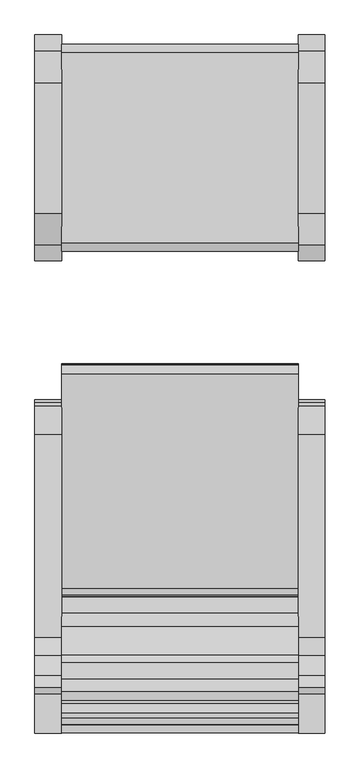
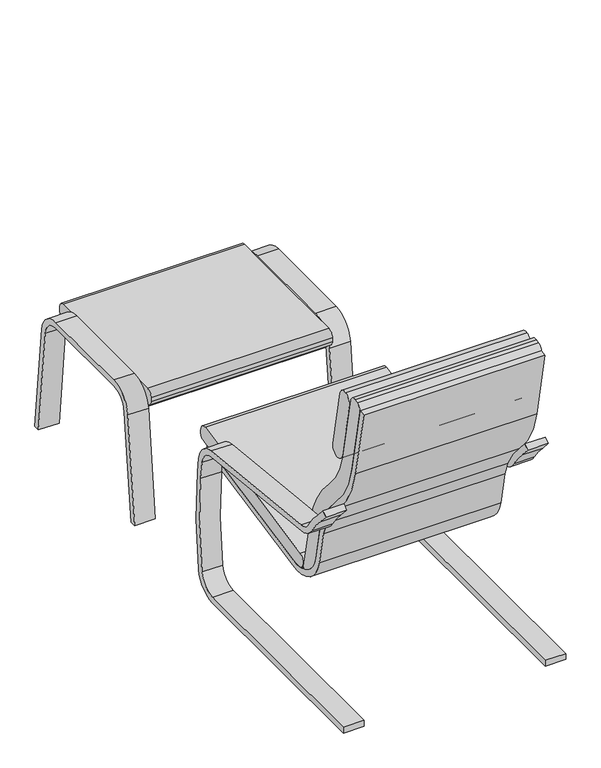
"""IFC4 building model written with IfcOpenShell, lengths in millimetres: furniture geometry."""

from ifc_helpers import new_model, si_unit, point, frame, frame_2d, origin, place, context, project, spatial, polyline, circle_curve, trimmed, segment, composite_curve, outline, extrude, source, transform, mapped, element, save


def furniture_b0964881(model_context):
    return source(origin(), model_context, "Body", "SweptSolid", [
        extrude(outline(composite_curve([segment(polyline([(-419.1, 19.05), (279.4542155, 19.05)]), True, "CONTINUOUS"), segment(trimmed(circle_curve(frame_2d((279.4542155, 76.2)), 57.15), [point((279.4542155, 19.05))], [point((335.932198, 67.4615796))], True, "CARTESIAN"), True, "CONTINUOUS"), segment(trimmed(circle_curve(frame_2d((-796.2501085, 242.6357718)), 1145.6538626), [point((335.932198, 67.4615796))], [point((342.5646303, 367.6308255))], True, "CARTESIAN"), True, "CONTINUOUS"), segment(trimmed(circle_curve(frame_2d((-796.2501085, 242.6357718)), 1145.6538626), [point((342.5646303, 367.6308255))], [point((334.8764989, 424.5021261))], True, "CARTESIAN"), True, "CONTINUOUS"), segment(trimmed(circle_curve(frame_2d((278.4511791, 415.4298727)), 57.15), [point((334.8764989, 424.5021261))], [point((284.4291769, 472.2663579))], True, "CARTESIAN"), True, "CONTINUOUS"), segment(polyline([(284.4291769, 472.2663579), (-194.9045529, 522.682143)]), True, "CONTINUOUS"), segment(trimmed(circle_curve(frame_2d((-186.9338891, 598.4641231)), 76.2), [point((-194.9045529, 522.682143))], [point((-251.8204957, 558.5120484))], False, "CARTESIAN"), True, "CONTINUOUS"), segment(trimmed(circle_curve(frame_2d((-499.260365, 406.1580161)), 290.5825873), [point((-251.8204957, 558.5120484))], [point((-296.3293666, 614.1417893))], True, "CARTESIAN"), True, "CONTINUOUS"), segment(trimmed(circle_curve(frame_2d((-56.8620262, 859.5716222)), 342.9), [point((-296.3293666, 614.1417893))], [point((-326.0096311, 647.1099157))], False, "CARTESIAN"), True, "CONTINUOUS"), segment(polyline([(-326.0096311, 647.1099157), (-311.0569864, 658.9133438)]), True, "CONTINUOUS"), segment(trimmed(circle_curve(frame_2d((-56.8620262, 859.5716222)), 323.85), [point((-311.0569864, 658.9133438))], [point((-283.0256254, 627.7767801))], True, "CARTESIAN"), True, "CONTINUOUS"), segment(trimmed(circle_curve(frame_2d((-499.260365, 406.1580161)), 309.6325873), [point((-283.0256254, 627.7767801))], [point((-235.598844, 568.500067))], False, "CARTESIAN"), True, "CONTINUOUS"), segment(trimmed(circle_curve(frame_2d((-186.9338891, 598.4641231)), 57.15), [point((-235.598844, 568.500067))], [point((-192.9118869, 541.627638))], True, "CARTESIAN"), True, "CONTINUOUS"), segment(polyline([(-192.9118869, 541.627638), (286.4218429, 491.2118529)]), True, "CONTINUOUS"), segment(trimmed(circle_curve(frame_2d((278.4511791, 415.4298727)), 76.2), [point((286.4218429, 491.2118529))], [point((353.6849388, 427.5262106))], False, "CARTESIAN"), True, "CONTINUOUS"), segment(trimmed(circle_curve(frame_2d((-796.2501085, 242.6357718)), 1164.7038626), [point((353.6849388, 427.5262106))], [point((360.5049853, 378.4766361))], False, "CARTESIAN"), True, "CONTINUOUS"), segment(trimmed(circle_curve(frame_2d((-796.2501085, 242.6357718)), 1164.7038626), [point((360.5049853, 378.4766361))], [point((354.7581922, 64.5487728))], False, "CARTESIAN"), True, "CONTINUOUS"), segment(trimmed(circle_curve(frame_2d((279.4542155, 76.2)), 76.2), [point((354.7581922, 64.5487728))], [point((279.4542155, 0.0))], False, "CARTESIAN"), True, "CONTINUOUS"), segment(polyline([(279.4542155, 0.0), (-419.1, 0.0), (-419.1, 19.05)]), True, "CONTINUOUS")], self_intersect=False)), frame((279.4, 0.0, 0.0), z_axis=(1.0, 0.0, 0.0), x_axis=(0.0, 1.0, 0.0)), (0.0, 0.0, 1.0), 63.5),
        extrude(outline(composite_curve([segment(polyline([(-419.1, 19.05), (279.4542155, 19.05)]), True, "CONTINUOUS"), segment(trimmed(circle_curve(frame_2d((279.4542155, 76.2)), 57.15), [point((279.4542155, 19.05))], [point((335.932198, 67.4615796))], True, "CARTESIAN"), True, "CONTINUOUS"), segment(trimmed(circle_curve(frame_2d((-796.2501085, 242.6357718)), 1145.6538626), [point((335.932198, 67.4615796))], [point((342.5646303, 367.6308255))], True, "CARTESIAN"), True, "CONTINUOUS"), segment(trimmed(circle_curve(frame_2d((-796.2501085, 242.6357718)), 1145.6538626), [point((342.5646303, 367.6308255))], [point((334.8764989, 424.5021261))], True, "CARTESIAN"), True, "CONTINUOUS"), segment(trimmed(circle_curve(frame_2d((278.4511791, 415.4298727)), 57.15), [point((334.8764989, 424.5021261))], [point((284.4291769, 472.2663579))], True, "CARTESIAN"), True, "CONTINUOUS"), segment(polyline([(284.4291769, 472.2663579), (-194.9045529, 522.682143)]), True, "CONTINUOUS"), segment(trimmed(circle_curve(frame_2d((-186.9338891, 598.4641231)), 76.2), [point((-194.9045529, 522.682143))], [point((-251.8204957, 558.5120484))], False, "CARTESIAN"), True, "CONTINUOUS"), segment(trimmed(circle_curve(frame_2d((-499.260365, 406.1580161)), 290.5825873), [point((-251.8204957, 558.5120484))], [point((-296.3293666, 614.1417893))], True, "CARTESIAN"), True, "CONTINUOUS"), segment(trimmed(circle_curve(frame_2d((-56.8620262, 859.5716222)), 342.9), [point((-296.3293666, 614.1417893))], [point((-326.0096311, 647.1099157))], False, "CARTESIAN"), True, "CONTINUOUS"), segment(polyline([(-326.0096311, 647.1099157), (-311.0569864, 658.9133438)]), True, "CONTINUOUS"), segment(trimmed(circle_curve(frame_2d((-56.8620262, 859.5716222)), 323.85), [point((-311.0569864, 658.9133438))], [point((-283.0256254, 627.7767801))], True, "CARTESIAN"), True, "CONTINUOUS"), segment(trimmed(circle_curve(frame_2d((-499.260365, 406.1580161)), 309.6325873), [point((-283.0256254, 627.7767801))], [point((-235.598844, 568.500067))], False, "CARTESIAN"), True, "CONTINUOUS"), segment(trimmed(circle_curve(frame_2d((-186.9338891, 598.4641231)), 57.15), [point((-235.598844, 568.500067))], [point((-192.9118869, 541.627638))], True, "CARTESIAN"), True, "CONTINUOUS"), segment(polyline([(-192.9118869, 541.627638), (286.4218429, 491.2118529)]), True, "CONTINUOUS"), segment(trimmed(circle_curve(frame_2d((278.4511791, 415.4298727)), 76.2), [point((286.4218429, 491.2118529))], [point((353.6849388, 427.5262106))], False, "CARTESIAN"), True, "CONTINUOUS"), segment(trimmed(circle_curve(frame_2d((-796.2501085, 242.6357718)), 1164.7038626), [point((353.6849388, 427.5262106))], [point((360.5049853, 378.4766361))], False, "CARTESIAN"), True, "CONTINUOUS"), segment(trimmed(circle_curve(frame_2d((-796.2501085, 242.6357718)), 1164.7038626), [point((360.5049853, 378.4766361))], [point((354.7581922, 64.5487728))], False, "CARTESIAN"), True, "CONTINUOUS"), segment(trimmed(circle_curve(frame_2d((279.4542155, 76.2)), 76.2), [point((354.7581922, 64.5487728))], [point((279.4542155, 0.0))], False, "CARTESIAN"), True, "CONTINUOUS"), segment(polyline([(279.4542155, 0.0), (-419.1, 0.0), (-419.1, 19.05)]), True, "CONTINUOUS")], self_intersect=False)), frame((-342.9, 0.0, 0.0), z_axis=(1.0, 0.0, 0.0), x_axis=(0.0, 1.0, 0.0)), (0.0, 0.0, 1.0), 63.5),
        extrude(outline(composite_curve([segment(polyline([(-42.5349168, 312.6304075), (419.1, 406.4), (422.8920916, 387.7312416), (-38.7428252, 293.9616491)]), True, "CONTINUOUS"), segment(trimmed(circle_curve(frame_2d((-62.7594051, 412.1971192)), 120.65), [point((-38.7428252, 293.9616491))], [point((-180.9948752, 388.1805393))], False, "CARTESIAN"), True, "CONTINUOUS"), segment(polyline([(-180.9948752, 388.1805393), (-202.7876044, 495.4678216)]), True, "CONTINUOUS"), segment(trimmed(circle_curve(frame_2d((-499.260365, 406.1580161)), 309.6325873), [point((-202.7876044, 495.4678216))], [point((-220.9693132, 541.9020016))], True, "CARTESIAN"), True, "CONTINUOUS"), segment(trimmed(circle_curve(frame_2d((-499.260365, 406.1580161)), 309.6325873), [point((-220.9693132, 541.9020016))], [point((-283.0256254, 627.7767801))], True, "CARTESIAN"), True, "CONTINUOUS"), segment(trimmed(circle_curve(frame_2d((-56.8620262, 859.5716222)), 323.85), [point((-283.0256254, 627.7767801))], [point((-374.2309196, 795.1060658))], False, "CARTESIAN"), True, "CONTINUOUS"), segment(polyline([(-374.2309196, 795.1060658), (-418.3297314, 1012.2079084), (-399.660973, 1016.0), (-355.5621612, 798.8981573)]), True, "CONTINUOUS"), segment(trimmed(circle_curve(frame_2d((-56.8620262, 859.5716222)), 304.8), [point((-355.5621612, 798.8981573))], [point((-269.7218843, 641.4117708))], True, "CARTESIAN"), True, "CONTINUOUS"), segment(trimmed(circle_curve(frame_2d((-499.260365, 406.1580161)), 328.6825873), [point((-269.7218843, 641.4117708))], [point((-194.9403545, 530.341648))], False, "CARTESIAN"), True, "CONTINUOUS"), segment(trimmed(circle_curve(frame_2d((-499.260365, 406.1580161)), 328.6825873), [point((-194.9403545, 530.341648))], [point((-184.2911624, 500.1082404))], False, "CARTESIAN"), True, "CONTINUOUS"), segment(polyline([(-184.2911624, 500.1082404), (-162.3261167, 391.9726309)]), True, "CONTINUOUS"), segment(trimmed(circle_curve(frame_2d((-62.7594051, 412.1971192)), 101.6), [point((-162.3261167, 391.9726309))], [point((-42.5349168, 312.6304075))], True, "CARTESIAN"), True, "CONTINUOUS")], self_intersect=False)), frame((-279.4, 0.0, 0.0), z_axis=(1.0, 0.0, 0.0), x_axis=(0.0, 1.0, 0.0)), (0.0, 0.0, 1.0), 558.8),
        extrude(outline(composite_curve([segment(trimmed(circle_curve(frame_2d((-62.7594051, 412.1971192)), 101.6), [point((-99.3910669, 317.4306623))], [point((-162.3261167, 391.9726309))], False, "CARTESIAN"), True, "CONTINUOUS"), segment(polyline([(-162.3261167, 391.9726309), (-184.2911624, 500.1082404)]), True, "CONTINUOUS"), segment(trimmed(circle_curve(frame_2d((-499.260365, 406.1580161)), 328.6825873), [point((-184.2911624, 500.1082404))], [point((-194.9403545, 530.341648))], True, "CARTESIAN"), True, "CONTINUOUS"), segment(trimmed(circle_curve(frame_2d((-499.260365, 406.1580161)), 328.6825873), [point((-194.9403545, 530.341648))], [point((-269.7218843, 641.4117708))], True, "CARTESIAN"), True, "CONTINUOUS"), segment(trimmed(circle_curve(frame_2d((-56.8620262, 859.5716222)), 304.8), [point((-269.7218843, 641.4117708))], [point((-355.5621612, 798.8981573))], False, "CARTESIAN"), True, "CONTINUOUS"), segment(polyline([(-355.5621612, 798.8981573), (-398.3969424, 1009.7770805)]), True, "CONTINUOUS"), segment(trimmed(circle_curve(frame_2d((-379.728184, 1013.5691721)), 19.05), [point((-398.3969424, 1009.7770805))], [point((-383.5202756, 1032.2379305))], False, "CARTESIAN"), True, "CONTINUOUS"), segment(polyline([(-383.5202756, 1032.2379305), (-371.0744366, 1034.7659916)]), True, "CONTINUOUS"), segment(trimmed(circle_curve(frame_2d((-367.282345, 1016.0972331)), 19.05), [point((-371.0744366, 1034.7659916))], [point((-348.6135866, 1019.8893247))], False, "CARTESIAN"), True, "CONTINUOUS"), segment(polyline([(-348.6135866, 1019.8893247), (-305.7788053, 809.0104015)]), True, "CONTINUOUS"), segment(trimmed(circle_curve(frame_2d((-56.8620262, 859.5716222)), 254.0), [point((-305.7788053, 809.0104015))], [point((-234.2452413, 677.771746))], True, "CARTESIAN"), True, "CONTINUOUS"), segment(trimmed(circle_curve(frame_2d((-499.260365, 406.1580161)), 379.4825873), [point((-234.2452413, 677.771746))], [point((-167.2898954, 590.0129627))], False, "CARTESIAN"), True, "CONTINUOUS"), segment(trimmed(circle_curve(frame_2d((-499.260365, 406.1580161)), 379.4825873), [point((-167.2898954, 590.0129627))], [point((-134.9442561, 512.3691591))], False, "CARTESIAN"), True, "CONTINUOUS"), segment(polyline([(-134.9442561, 512.3691591), (-97.1938516, 326.5210137)]), True, "CONTINUOUS"), segment(trimmed(circle_curve(frame_2d((-110.4043038, 324.903374)), 13.309125), [point((-97.1938516, 326.5210137))], [point((-99.3910669, 317.4306623))], False, "CARTESIAN"), True, "CONTINUOUS")], self_intersect=False)), frame((-279.4, 0.0, 0.0), z_axis=(1.0, 0.0, 0.0), x_axis=(0.0, 1.0, 0.0)), (0.0, 0.0, 1.0), 558.8),
        extrude(outline(composite_curve([segment(polyline([(-303.0807625, 811.7084443), (-340.8594217, 997.6956896)]), True, "CONTINUOUS"), segment(trimmed(circle_curve(frame_2d((-315.9677438, 1002.7518117)), 25.4), [point((-340.8594217, 997.6956896))], [point((-321.0238659, 1027.6434896))], False, "CARTESIAN"), True, "CONTINUOUS"), segment(trimmed(circle_curve(frame_2d((-315.9677438, 1002.7518117)), 25.4), [point((-321.0238659, 1027.6434896))], [point((-291.0760659, 1007.8079337))], False, "CARTESIAN"), True, "CONTINUOUS"), segment(polyline([(-291.0760659, 1007.8079337), (-253.2974067, 821.8206885)]), True, "CONTINUOUS"), segment(trimmed(circle_curve(frame_2d((-278.1890846, 816.7645664)), 25.4), [point((-253.2974067, 821.8206885))], [point((-273.1329625, 791.8728885))], False, "CARTESIAN"), True, "CONTINUOUS"), segment(trimmed(circle_curve(frame_2d((-278.1890846, 816.7645664)), 25.4), [point((-273.1329625, 791.8728885))], [point((-303.0807625, 811.7084443))], False, "CARTESIAN"), True, "CONTINUOUS")], self_intersect=False)), frame((-279.4, 0.0, 0.0), z_axis=(1.0, 0.0, 0.0), x_axis=(0.0, 1.0, 0.0)), (0.0, 0.0, 1.0), 558.8),
        extrude(outline(composite_curve([segment(polyline([(-77.5388388, 357.3576413), (427.6565143, 459.9754474)]), True, "CONTINUOUS"), segment(trimmed(circle_curve(frame_2d((431.4486058, 441.306689)), 19.05), [point((427.6565143, 459.9754474))], [point((450.1173643, 445.0987805))], False, "CARTESIAN"), True, "CONTINUOUS"), segment(polyline([(450.1173643, 445.0987805), (452.6454253, 432.6529416)]), True, "CONTINUOUS"), segment(trimmed(circle_curve(frame_2d((433.9766669, 428.86085)), 19.05), [point((452.6454253, 432.6529416))], [point((437.7687584, 410.1920916))], False, "CARTESIAN"), True, "CONTINUOUS"), segment(polyline([(437.7687584, 410.1920916), (-42.5349168, 312.6304075)]), True, "CONTINUOUS"), segment(trimmed(circle_curve(frame_2d((-62.7594051, 412.1971192)), 101.6), [point((-42.5349168, 312.6304075))], [point((-84.9638595, 313.0531723))], False, "CARTESIAN"), True, "CONTINUOUS"), segment(trimmed(circle_curve(frame_2d((-71.2186862, 326.2430439)), 19.05), [point((-84.9638595, 313.0531723))], [point((-89.8874447, 322.4509523))], False, "CARTESIAN"), True, "CONTINUOUS"), segment(polyline([(-89.8874447, 322.4509523), (-92.4155057, 334.8967913)]), True, "CONTINUOUS"), segment(trimmed(circle_curve(frame_2d((-73.7467473, 338.6888829)), 19.05), [point((-92.4155057, 334.8967913))], [point((-77.5388388, 357.3576413))], False, "CARTESIAN"), True, "CONTINUOUS")], self_intersect=False)), frame((-279.4, 0.0, 0.0), z_axis=(1.0, 0.0, 0.0), x_axis=(0.0, 1.0, 0.0)), (0.0, 0.0, 1.0), 558.8),
        extrude(outline(composite_curve([segment(polyline([(1192.1548456, 338.42809), (1228.9132979, 0.0), (1209.7512584, 0.0), (1173.21623, 336.3710675)]), True, "CONTINUOUS"), segment(trimmed(circle_curve(frame_2d((1116.4003834, 330.2)), 57.15), [point((1173.21623, 336.3710675))], [point((1116.4003834, 387.35))], True, "CARTESIAN"), True, "CONTINUOUS"), segment(polyline([(1116.4003834, 387.35), (808.0262124, 387.35)]), True, "CONTINUOUS"), segment(trimmed(circle_curve(frame_2d((808.0262124, 330.2)), 57.15), [point((808.0262124, 387.35))], [point((751.2103658, 336.3710675))], True, "CARTESIAN"), True, "CONTINUOUS"), segment(polyline([(751.2103658, 336.3710675), (714.6753375, 0.0), (695.5132979, 0.0), (732.2717503, 338.42809)]), True, "CONTINUOUS"), segment(trimmed(circle_curve(frame_2d((808.0262124, 330.2)), 76.2), [point((732.2717503, 338.42809))], [point((808.0262124, 406.4))], False, "CARTESIAN"), True, "CONTINUOUS"), segment(polyline([(808.0262124, 406.4), (1116.4003834, 406.4)]), True, "CONTINUOUS"), segment(trimmed(circle_curve(frame_2d((1116.4003834, 330.2)), 76.2), [point((1116.4003834, 406.4))], [point((1192.1548456, 338.42809))], False, "CARTESIAN"), True, "CONTINUOUS")], self_intersect=False)), frame((279.4, 0.0, 0.0), z_axis=(1.0, 0.0, 0.0), x_axis=(0.0, 1.0, 0.0)), (0.0, 0.0, 1.0), 63.5),
        extrude(outline(composite_curve([segment(polyline([(1192.1548456, 338.42809), (1228.9132979, 0.0), (1209.7512584, 0.0), (1173.21623, 336.3710675)]), True, "CONTINUOUS"), segment(trimmed(circle_curve(frame_2d((1116.4003834, 330.2)), 57.15), [point((1173.21623, 336.3710675))], [point((1116.4003834, 387.35))], True, "CARTESIAN"), True, "CONTINUOUS"), segment(polyline([(1116.4003834, 387.35), (808.0262124, 387.35)]), True, "CONTINUOUS"), segment(trimmed(circle_curve(frame_2d((808.0262124, 330.2)), 57.15), [point((808.0262124, 387.35))], [point((751.2103658, 336.3710675))], True, "CARTESIAN"), True, "CONTINUOUS"), segment(polyline([(751.2103658, 336.3710675), (714.6753375, 0.0), (695.5132979, 0.0), (732.2717503, 338.42809)]), True, "CONTINUOUS"), segment(trimmed(circle_curve(frame_2d((808.0262124, 330.2)), 76.2), [point((732.2717503, 338.42809))], [point((808.0262124, 406.4))], False, "CARTESIAN"), True, "CONTINUOUS"), segment(polyline([(808.0262124, 406.4), (1116.4003834, 406.4)]), True, "CONTINUOUS"), segment(trimmed(circle_curve(frame_2d((1116.4003834, 330.2)), 76.2), [point((1116.4003834, 406.4))], [point((1192.1548456, 338.42809))], False, "CARTESIAN"), True, "CONTINUOUS")], self_intersect=False)), frame((-342.9, 0.0, 0.0), z_axis=(1.0, 0.0, 0.0), x_axis=(0.0, 1.0, 0.0)), (0.0, 0.0, 1.0), 63.5),
        extrude(outline(composite_curve([segment(trimmed(circle_curve(frame_2d((1187.3562224, 368.3)), 19.05), [point((1206.4062224, 368.3))], [point((1187.3562224, 349.25))], False, "CARTESIAN"), True, "CONTINUOUS"), segment(polyline([(1187.3562224, 349.25), (737.0703734, 349.25)]), True, "CONTINUOUS"), segment(trimmed(circle_curve(frame_2d((737.0703734, 368.3)), 19.05), [point((737.0703734, 349.25))], [point((718.0203734, 368.3))], False, "CARTESIAN"), True, "CONTINUOUS"), segment(polyline([(718.0203734, 368.3), (718.0203734, 381.0)]), True, "CONTINUOUS"), segment(trimmed(circle_curve(frame_2d((737.0703734, 381.0)), 19.05), [point((718.0203734, 381.0))], [point((737.0703734, 400.05))], False, "CARTESIAN"), True, "CONTINUOUS"), segment(polyline([(737.0703734, 400.05), (1187.3562224, 400.05)]), True, "CONTINUOUS"), segment(trimmed(circle_curve(frame_2d((1187.3562224, 381.0)), 19.05), [point((1187.3562224, 400.05))], [point((1206.4062224, 381.0))], False, "CARTESIAN"), True, "CONTINUOUS"), segment(polyline([(1206.4062224, 381.0), (1206.4062224, 368.3)]), True, "CONTINUOUS")], self_intersect=False)), frame((-279.4, 0.0, 0.0), z_axis=(1.0, 0.0, 0.0), x_axis=(0.0, 1.0, 0.0)), (0.0, 0.0, 1.0), 558.8),
        extrude(outline(composite_curve([segment(trimmed(circle_curve(frame_2d((1116.4003834, 330.2)), 57.15), [point((1170.2819202, 349.25))], [point((1173.21623, 336.3710675))], False, "CARTESIAN"), True, "CONTINUOUS"), segment(polyline([(1173.21623, 336.3710675), (1173.8865021, 330.2), (750.5400937, 330.2), (751.2103658, 336.3710675)]), True, "CONTINUOUS"), segment(trimmed(circle_curve(frame_2d((808.0262124, 330.2)), 57.15), [point((751.2103658, 336.3710675))], [point((754.1446757, 349.25))], False, "CARTESIAN"), True, "CONTINUOUS"), segment(polyline([(754.1446757, 349.25), (1170.2819202, 349.25)]), True, "CONTINUOUS")], self_intersect=False)), frame((-279.4, 0.0, 0.0), z_axis=(1.0, 0.0, 0.0), x_axis=(0.0, 1.0, 0.0)), (0.0, 0.0, 1.0), 558.8),
    ])


if __name__ == "__main__":
    model = new_model("IFC4")
    model_context = context("Model", 3, world=origin())
    ifc_project = project(units=[si_unit("LENGTHUNIT", "METRE", prefix="MILLI")], contexts=[model_context])
    site = spatial("IfcSite", under=ifc_project)
    building = spatial("IfcBuilding", under=site)
    placement = place(None, origin())
    furniture_shape = furniture_b0964881(model_context)
    element("IfcFurniture", 1, at=placement, inside=building, context=model_context, shape_type="MappedRepresentation", body=[
        mapped(furniture_shape, transform((0.0, 0.0, 0.0), x_axis=(1.0, 0.0, 0.0), y_axis=(0.0, 1.0, 0.0), z_axis=(0.0, 0.0, 1.0))),
    ])
    save(model, "model.ifc")

# Revit data of these elements
# Type
#   Default Elevation = 0
# Element 1 (IfcFurniture)
#   Materials on its faces: "Wood", "cushion"
# Materials
#   "Wood": class "Wood", colour RGB 212 179 113, transparency 0, Description = "Generic wood", Cost = 0
#   "cushion": class "Fabric", colour RGB 78 81 77, transparency 0
